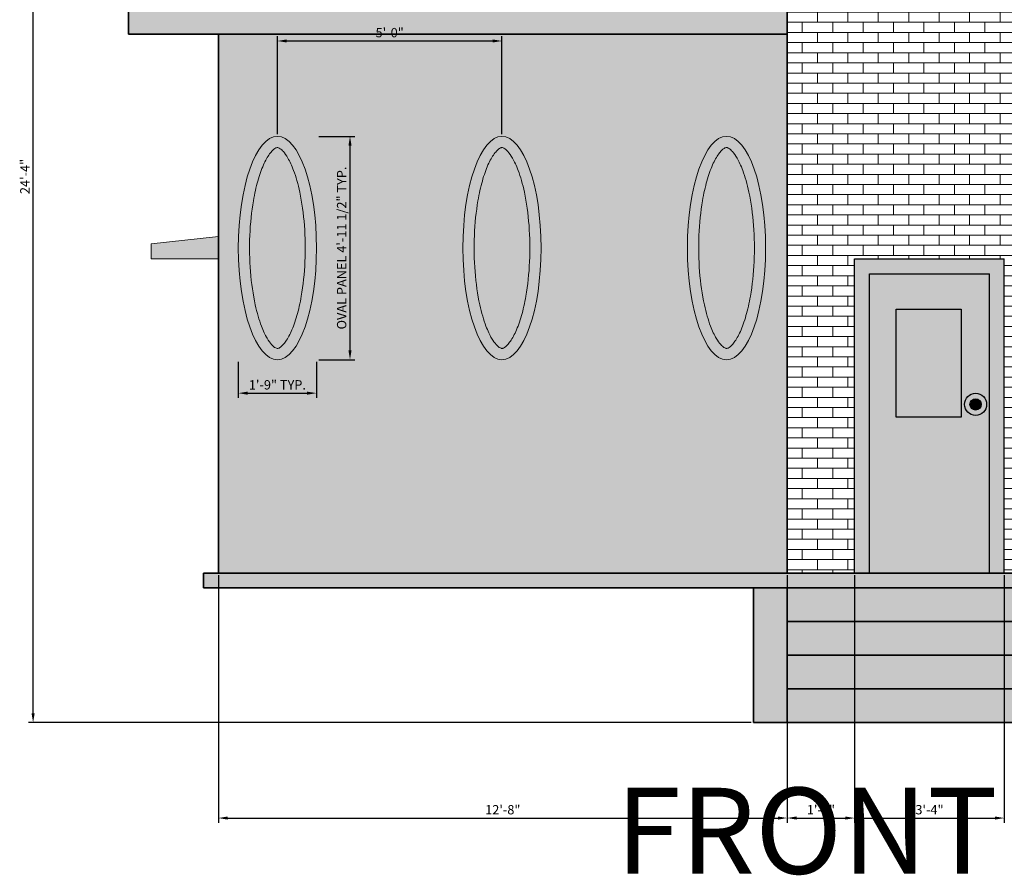
# Model space of a CAD drawing. Units: inches. Extents: x 4878 to 9282, y 5367 to 6617.
# Tile 1 of 14: x 4936 to 5199, y 5367 to 5596. Entities that reach past the tile are written whole.
import ezdxf

# ---------------------------------------------------------------- set-up
doc = ezdxf.new("R2010")
doc.units = ezdxf.units.IN
for name, color, linetype, lineweight in [('A-ANNO-DIMS', 2, 'Continuous', 18), ('A-ANNO-TITL', 3, 'Continuous', 30), ('A-ELEV', 7, 'Continuous', 35), ('A-ELEV-DOOR', 3, 'Continuous', 25), ('A-ELEV-TRIM', 7, 'Continuous', 20)]:
    doc.layers.add(name, color=color, linetype=linetype, lineweight=lineweight)
for name, color, linetype, lineweight, true_color in [('A-ELEV-BASE-PATT', 252, 'Continuous', 13, 0x939598), ('A-ELEV-CLAD-PATT', 215, 'Continuous', 13, 0xa953a0), ('A-ELEV-DOOR-PATT', 37, 'Continuous', 13, 0x7f5f3f), ('A-ELEV-METL-PATT', 252, 'Continuous', 13, 0x939598), ('A-ELEV-PANL-PATT', 41, 'Continuous', 13, 0xf4ee51), ('A-ELEV-TRIM-PATT', 11, 'Continuous', 13, 0xf27172), ('A-ELEV-WALL-PATT', 9, 'Continuous', 13, 0xafd9aa)]:
    doc.layers.add(name, color=color, linetype=linetype, lineweight=lineweight, true_color=true_color)
doc.styles.get("Standard").update_dxf_attribs({"font": 'arial.ttf'})
doc.dimstyles.new('ISO-25', dxfattribs={"dimtxt": 2.5, "dimasz": 2.5, "dimexe": 1.25, "dimexo": 0.625, "dimtad": 1, "dimdec": 0, "dimlunit": 3, "dimtxsty": 'Standard', "dimcen": 2.5, "dimadec": 0, "dimazin": 0, "dimtfac": 1, "dimtdec": 0, "dimtmove": 0, "dimatfit": 3, "dimfxl": 1, "dimarcsym": 0})

# ---------------------------------------------------------------- blocks, each defined once
blk = doc.blocks.new('FACADE-OVAL-PANEL')
blk.add_ellipse((10.45, 29.85), major_axis=(0, -29.85), ratio=0.35)
blk.add_open_spline([(10.45, 3), (10.51, 3), (10.59, 3.01), (10.8, 3.08), (10.94, 3.14), (11.29, 3.36), (11.5, 3.53), (11.97, 3.99), (12.23, 4.29), (13.03, 5.37), (13.6, 6.35), (14.68, 8.75), (15.19, 10.18), (16.1, 13.36), (16.5, 15.12), (17.33, 19.86), (17.67, 23), (17.95, 29.42), (17.91, 32.7), (17.43, 39.02), (17.01, 42.06), (15.97, 46.94), (15.4, 48.9), (14.3, 51.87), (13.77, 52.99), (12.83, 54.61), (12.41, 55.2), (11.72, 55.97), (11.44, 56.22), (11.01, 56.52), (10.85, 56.6), (10.62, 56.68), (10.54, 56.69), (10.39, 56.7), (10.32, 56.69), (10.11, 56.63), (9.97, 56.57), (9.61, 56.34), (9.39, 56.16), (8.9, 55.68), (8.63, 55.37), (7.82, 54.26), (7.25, 53.26), (6.17, 50.82), (5.65, 49.37), (4.75, 46.15), (4.35, 44.37), (3.53, 39.59), (3.2, 36.44), (2.94, 30), (3, 26.71), (3.49, 20.39), (3.93, 17.36), (4.99, 12.53), (5.55, 10.61), (6.65, 7.7), (7.17, 6.6), (8.1, 5.01), (8.52, 4.45), (9.2, 3.69), (9.48, 3.45), (9.94, 3.14), (10.11, 3.07), (10.32, 3.01), (10.38, 3), (10.45, 3)], degree=3, knots=[0, 0, 0, 0, 0.110339, 0.110339, 0.220677, 0.220677, 0.331016, 0.331016, 0.441355, 0.441355, 0.663086, 0.663086, 0.884817, 0.884817, 1.106548, 1.106548, 1.444005, 1.444005, 1.781462, 1.781462, 2.118918, 2.118918, 2.388345, 2.388345, 2.598365, 2.598365, 2.76649, 2.76649, 2.902512, 2.902512, 3.016819, 3.016819, 3.131125, 3.131125, 3.245431, 3.245431, 3.359737, 3.359737, 3.474044, 3.474044, 3.58835, 3.58835, 3.811147, 3.811147, 4.033944, 4.033944, 4.256741, 4.256741, 4.594929, 4.594929, 4.933117, 4.933117, 5.271305, 5.271305, 5.538007, 5.538007, 5.746376, 5.746376, 5.91327, 5.91327, 6.048323, 6.048323, 6.183376, 6.183376, 6.283185, 6.283185, 6.283185, 6.283185])
blk = doc.blocks.new('*D49')
at = {"layer": 'A-ANNO-DIMS', "color": 0, "lineweight": -2, "transparency": 16777216}
for p, q in [((5015.83, 5564.48), (5025.4, 5564.48)), ((5024.15, 5507.29), (5024.15, 5561.98)), ((5015.83, 5504.79), (5025.4, 5504.79))]:
    blk.add_line(p, q, dxfattribs=at)
at = {"layer": 'A-ANNO-DIMS', "color": 0, "transparency": 16777216}
for points in [[(5023.74, 5561.98), (5024.57, 5561.98), (5024.15, 5564.48)], [(5023.74, 5507.29), (5024.57, 5507.29), (5024.15, 5504.79)]]:
    blk.add_solid(points, dxfattribs=at)
at = {"layer": 'Defpoints', "color": 0, "transparency": 16777216}
for p in [(5015.2, 5564.48), (5024.15, 5564.48), (5015.2, 5504.79)]:
    blk.add_point(p, dxfattribs=at)
at = {"layer": 'A-ANNO-DIMS', "color": 0, "transparency": 16777216, "insert": (5022.24, 5534.64), "char_height": 2.5, "attachment_point": 5, "rotation": 90}
blk.add_mtext('OVAL PANEL 4\'-11 1/2" TYP.', dxfattribs=at)
blk = doc.blocks.new('*D50')
at = {"layer": 'A-ANNO-DIMS', "color": 0, "lineweight": -2, "transparency": 16777216}
for p, q in [((4994.31, 5504.17), (4994.31, 5494.59)), ((5015.2, 5504.17), (5015.2, 5494.59)), ((4996.81, 5495.84), (5012.7, 5495.84))]:
    blk.add_line(p, q, dxfattribs=at)
at = {"layer": 'A-ANNO-DIMS', "color": 0, "transparency": 16777216}
for points in [[(4996.81, 5496.25), (4996.81, 5495.42), (4994.31, 5495.84)], [(5012.7, 5496.25), (5012.7, 5495.42), (5015.2, 5495.84)]]:
    blk.add_solid(points, dxfattribs=at)
at = {"layer": 'Defpoints', "color": 0, "transparency": 16777216}
for p in [(4994.31, 5504.79), (5015.2, 5504.79), (5015.2, 5495.84)]:
    blk.add_point(p, dxfattribs=at)
at = {"layer": 'A-ANNO-DIMS', "color": 0, "transparency": 16777216, "insert": (5004.75, 5497.74), "char_height": 2.5, "attachment_point": 5}
blk.add_mtext('1\'-9" TYP.', dxfattribs=at)
blk = doc.blocks.new('*D89')
at = {"layer": 'A-ANNO-DIMS', "color": 0, "lineweight": -2, "transparency": 16777216}
for p, q in [((5116.35, 5699.76), (4938.23, 5699.76)), ((4939.48, 5410.26), (4939.48, 5697.26)), ((5131.35, 5407.76), (4938.23, 5407.76))]:
    blk.add_line(p, q, dxfattribs=at)
at = {"layer": 'A-ANNO-DIMS', "color": 0, "transparency": 16777216}
for points in [[(4939.06, 5697.26), (4939.89, 5697.26), (4939.48, 5699.76)], [(4939.06, 5410.26), (4939.89, 5410.26), (4939.48, 5407.76)]]:
    blk.add_solid(points, dxfattribs=at)
at = {"layer": 'Defpoints', "color": 0, "transparency": 16777216}
for p in [(4939.48, 5699.76), (5116.98, 5699.76), (5131.98, 5407.76)]:
    blk.add_point(p, dxfattribs=at)
at = {"layer": 'A-ANNO-DIMS', "color": 0, "transparency": 16777216, "insert": (4937.6, 5553.76), "char_height": 2.5, "attachment_point": 5, "rotation": 90}
blk.add_mtext('24\'-4"', dxfattribs=at)
blk = doc.blocks.new('*D90')
at = {"layer": 'A-ANNO-DIMS', "color": 0, "lineweight": -2, "transparency": 16777216}
for p, q in [((4988.98, 5447.14), (4988.98, 5381.01)), ((5140.98, 5447.14), (5140.98, 5381.01)), ((4991.48, 5382.26), (5138.48, 5382.26))]:
    blk.add_line(p, q, dxfattribs=at)
at = {"layer": 'A-ANNO-DIMS', "color": 0, "transparency": 16777216}
for points in [[(4991.48, 5382.68), (4991.48, 5381.84), (4988.98, 5382.26)], [(5138.48, 5382.68), (5138.48, 5381.84), (5140.98, 5382.26)]]:
    blk.add_solid(points, dxfattribs=at)
at = {"layer": 'Defpoints', "color": 0, "transparency": 16777216}
for p in [(4988.98, 5447.76), (5140.98, 5447.76), (5140.98, 5382.26)]:
    blk.add_point(p, dxfattribs=at)
at = {"layer": 'A-ANNO-DIMS', "color": 0, "transparency": 16777216, "insert": (5064.98, 5384.16), "char_height": 2.5, "attachment_point": 5}
blk.add_mtext('12\'-8"', dxfattribs=at)
blk = doc.blocks.new('*D91')
at = {"layer": 'A-ANNO-DIMS', "color": 0, "lineweight": -2, "transparency": 16777216}
for p, q in [((5140.98, 5447.14), (5140.98, 5381.01)), ((5158.98, 5447.14), (5158.98, 5381.01)), ((5143.48, 5382.26), (5156.48, 5382.26))]:
    blk.add_line(p, q, dxfattribs=at)
at = {"layer": 'A-ANNO-DIMS', "color": 0, "transparency": 16777216}
for points in [[(5143.48, 5382.68), (5143.48, 5381.84), (5140.98, 5382.26)], [(5156.48, 5382.68), (5156.48, 5381.84), (5158.98, 5382.26)]]:
    blk.add_solid(points, dxfattribs=at)
at = {"layer": 'Defpoints', "color": 0, "transparency": 16777216}
for p in [(5140.98, 5447.76), (5158.98, 5447.76), (5158.98, 5382.26)]:
    blk.add_point(p, dxfattribs=at)
at = {"layer": 'A-ANNO-DIMS', "color": 0, "transparency": 16777216, "insert": (5149.98, 5384.16), "char_height": 2.5, "attachment_point": 5}
blk.add_mtext('1\'-6"', dxfattribs=at)
blk = doc.blocks.new('*D92')
at = {"layer": 'A-ANNO-DIMS', "color": 0, "lineweight": -2, "transparency": 16777216}
for p, q in [((5158.98, 5447.14), (5158.98, 5381.01)), ((5198.98, 5447.14), (5198.98, 5381.01)), ((5161.48, 5382.26), (5196.48, 5382.26))]:
    blk.add_line(p, q, dxfattribs=at)
at = {"layer": 'A-ANNO-DIMS', "color": 0, "transparency": 16777216}
for points in [[(5161.48, 5382.68), (5161.48, 5381.84), (5158.98, 5382.26)], [(5196.48, 5382.68), (5196.48, 5381.84), (5198.98, 5382.26)]]:
    blk.add_solid(points, dxfattribs=at)
at = {"layer": 'Defpoints', "color": 0, "transparency": 16777216}
for p in [(5158.98, 5447.76), (5198.98, 5447.76), (5198.98, 5382.26)]:
    blk.add_point(p, dxfattribs=at)
at = {"layer": 'A-ANNO-DIMS', "color": 0, "transparency": 16777216, "insert": (5178.98, 5384.16), "char_height": 2.5, "attachment_point": 5}
blk.add_mtext('3\'-4"', dxfattribs=at)
blk = doc.blocks.new('*D99')
at = {"layer": 'A-ANNO-DIMS', "color": 0, "lineweight": -2, "transparency": 16777216}
for p, q in [((5004.75, 5565.11), (5004.75, 5591.23)), ((5064.75, 5565.11), (5064.75, 5591.23)), ((5007.25, 5589.98), (5062.25, 5589.98))]:
    blk.add_line(p, q, dxfattribs=at)
at = {"layer": 'A-ANNO-DIMS', "color": 0, "transparency": 16777216}
for points in [[(5007.25, 5590.4), (5007.25, 5589.57), (5004.75, 5589.98)], [(5062.25, 5590.4), (5062.25, 5589.57), (5064.75, 5589.98)]]:
    blk.add_solid(points, dxfattribs=at)
at = {"layer": 'Defpoints', "color": 0, "transparency": 16777216}
for p in [(5064.75, 5589.98), (5004.75, 5564.48), (5064.75, 5564.48)]:
    blk.add_point(p, dxfattribs=at)
at = {"layer": 'A-ANNO-DIMS', "color": 0, "transparency": 16777216, "insert": (5034.75, 5591.89), "char_height": 2.5, "attachment_point": 5}
blk.add_mtext('5\'-0"', dxfattribs=at)

msp = doc.modelspace()

# ---------------------------------------------------------------- hatches: boundary and pattern name
at = {"layer": 'A-ELEV-BASE-PATT'}
h = msp.add_hatch(color=256, dxfattribs=at)
h.dxf.hatch_style = 1
h.paths.add_polyline_path([(4984.98, 5447.76), (4984.98, 5443.76), (5449.48, 5443.76), (5449.48, 5447.76)])
h = msp.add_hatch(color=256, dxfattribs=at)
h.dxf.hatch_style = 1
h.paths.add_polyline_path([(5140.98, 5443.76), (5131.98, 5443.76), (5131.98, 5407.76), (5140.98, 5407.76)])
h.paths.add_polyline_path([(5302.48, 5407.76), (5311.48, 5407.76), (5311.48, 5443.76), (5302.48, 5443.76)])
h = msp.add_hatch(color=256, dxfattribs=at)
h.dxf.hatch_style = 1
h.paths.add_polyline_path([(5302.48, 5434.76), (5302.48, 5443.76), (5140.98, 5443.76), (5140.98, 5434.76)])
h.paths.add_polyline_path([(5302.48, 5416.76), (5302.48, 5425.76), (5140.98, 5425.76), (5140.98, 5416.76)])
h = msp.add_hatch(color=256, dxfattribs=at)
h.dxf.hatch_style = 1
h.paths.add_polyline_path([(5302.48, 5407.76), (5302.48, 5416.76), (5140.98, 5416.76), (5140.98, 5407.76)])
h.paths.add_polyline_path([(5140.98, 5434.76), (5140.98, 5425.76), (5302.48, 5425.76), (5302.48, 5434.76)])
at = {"layer": 'A-ELEV-CLAD-PATT'}
h = msp.add_hatch(dxfattribs=at)
h.set_pattern_fill('AR-BRSTD', color=256, scale=0.04)
h.set_pattern_definition([(0, (-2235.2307, 189.171), (0, 2.709672), []), (90, (-2235.2307, 189.171), (-4.064, 2.709672), [2.709672, -2.709672])])
h.paths.add_polyline_path([(5140.98, 5447.76), (5158.98, 5447.76), (5158.98, 5531.76), (5198.98, 5531.76), (5198.98, 5447.76), (5302.48, 5447.76), (5302.48, 5693.76), (5140.98, 5693.76)])
h.paths.add_polyline_path([(5225.95, 5537.76), (5279.95, 5537.76), (5279.95, 5531.76), (5273.95, 5531.76), (5273.95, 5495.76), (5231.95, 5495.76), (5231.95, 5531.76), (5225.95, 5531.76)], flags=16)
h.paths.add_polyline_path([(5234.95, 5528.76), (5270.95, 5528.76), (5270.95, 5498.76), (5234.95, 5498.76)], flags=0)
at = {"layer": 'A-ELEV-DOOR-PATT'}
h = msp.add_hatch(color=256, dxfattribs=at)
h.dxf.hatch_style = 1
h.paths.add_polyline_path([(5162.98, 5527.76), (5194.98, 5527.76), (5194.98, 5447.76), (5198.98, 5447.76), (5198.98, 5531.76), (5158.98, 5531.76), (5158.98, 5447.76), (5162.98, 5447.76)])
h.paths.add_polyline_path([(5170.08, 5489.4), (5187.41, 5489.4), (5187.41, 5518.26), (5170.08, 5518.26)], flags=17)
h = msp.add_hatch(color=256, dxfattribs=at)
h.dxf.hatch_style = 1
h.paths.add_polyline_path([(5162.98, 5527.76), (5162.98, 5447.76), (5194.98, 5447.76), (5194.98, 5527.76)])
h.paths.add_polyline_path([(5187.41, 5518.26), (5187.41, 5489.4), (5170.08, 5489.4), (5170.08, 5518.26)], flags=16)
h.paths.add_polyline_path([(5194.25, 5492.84, -1), (5188.34, 5492.84, -1)], flags=16)
h.paths.add_polyline_path([(5192.82, 5492.84, -1), (5189.78, 5492.84, -1)], flags=0)
at = {"layer": 'A-ELEV-METL-PATT'}
h = msp.add_hatch(color=256, dxfattribs=at)
h.dxf.hatch_style = 1
h.paths.add_polyline_path([(5188.34, 5492.84, 1), (5194.25, 5492.84, 1)])
h.paths.add_polyline_path([(5192.82, 5492.84, -1), (5189.78, 5492.84, -1)], flags=16)
h = msp.add_hatch(color=256, dxfattribs=at)
h.dxf.hatch_style = 1
h.paths.add_polyline_path([(5192.82, 5492.84, 1), (5189.78, 5492.84, 1)])
at = {"layer": 'A-ELEV-PANL-PATT'}
h = msp.add_hatch(color=256, dxfattribs=at)
h.dxf.hatch_style = 1
edge = h.paths.add_edge_path()
edge.add_spline(control_points=[(5004.75, 5507.79), (5004.82, 5507.79), (5004.89, 5507.8), (5005.1, 5507.87), (5005.24, 5507.93), (5005.6, 5508.15), (5005.81, 5508.32), (5006.28, 5508.78), (5006.54, 5509.08), (5007.34, 5510.16), (5007.91, 5511.14), (5008.99, 5513.54), (5009.5, 5514.97), (5010.41, 5518.15), (5010.81, 5519.91), (5011.64, 5524.65), (5011.98, 5527.79), (5012.26, 5534.21), (5012.21, 5537.49), (5011.74, 5543.82), (5011.32, 5546.85), (5010.27, 5551.73), (5009.71, 5553.69), (5008.6, 5556.66), (5008.08, 5557.78), (5007.14, 5559.41), (5006.72, 5559.99), (5006.03, 5560.76), (5005.75, 5561.01), (5005.32, 5561.31), (5005.16, 5561.39), (5004.92, 5561.47), (5004.85, 5561.48), (5004.7, 5561.49), (5004.63, 5561.48), (5004.42, 5561.42), (5004.28, 5561.36), (5003.92, 5561.13), (5003.7, 5560.96), (5003.21, 5560.47), (5002.94, 5560.16), (5002.12, 5559.05), (5001.55, 5558.05), (5000.47, 5555.61), (4999.96, 5554.17), (4999.05, 5550.94), (4998.66, 5549.16), (4997.84, 5544.38), (4997.51, 5541.23), (4997.24, 5534.79), (4997.3, 5531.5), (4997.8, 5525.18), (4998.24, 5522.15), (4999.29, 5517.32), (4999.86, 5515.4), (5000.96, 5512.49), (5001.48, 5511.39), (5002.41, 5509.8), (5002.83, 5509.24), (5003.51, 5508.48), (5003.79, 5508.24), (5004.24, 5507.93), (5004.42, 5507.86), (5004.63, 5507.8), (5004.69, 5507.79), (5004.75, 5507.79)], knot_values=[0, 0, 0, 0, 0.110339, 0.110339, 0.220677, 0.220677, 0.331016, 0.331016, 0.441355, 0.441355, 0.663086, 0.663086, 0.884817, 0.884817, 1.106548, 1.106548, 1.444005, 1.444005, 1.781462, 1.781462, 2.118918, 2.118918, 2.388345, 2.388345, 2.598365, 2.598365, 2.76649, 2.76649, 2.902512, 2.902512, 3.016819, 3.016819, 3.131125, 3.131125, 3.245431, 3.245431, 3.359737, 3.359737, 3.474044, 3.474044, 3.58835, 3.58835, 3.811147, 3.811147, 4.033944, 4.033944, 4.256741, 4.256741, 4.594929, 4.594929, 4.933117, 4.933117, 5.271305, 5.271305, 5.538007, 5.538007, 5.746376, 5.746376, 5.91327, 5.91327, 6.048323, 6.048323, 6.183376, 6.183376, 6.283185, 6.283185, 6.283185, 6.283185], degree=3, periodic=0)
edge = h.paths.add_edge_path()
edge.add_spline(control_points=[(5064.75, 5507.79), (5064.82, 5507.79), (5064.89, 5507.8), (5065.1, 5507.87), (5065.24, 5507.93), (5065.6, 5508.15), (5065.81, 5508.32), (5066.28, 5508.78), (5066.54, 5509.08), (5067.34, 5510.16), (5067.91, 5511.14), (5068.99, 5513.54), (5069.5, 5514.97), (5070.41, 5518.15), (5070.81, 5519.91), (5071.64, 5524.65), (5071.98, 5527.79), (5072.26, 5534.21), (5072.21, 5537.49), (5071.74, 5543.82), (5071.32, 5546.85), (5070.27, 5551.73), (5069.71, 5553.69), (5068.6, 5556.66), (5068.08, 5557.78), (5067.14, 5559.41), (5066.72, 5559.99), (5066.03, 5560.76), (5065.75, 5561.01), (5065.32, 5561.31), (5065.16, 5561.39), (5064.92, 5561.47), (5064.85, 5561.48), (5064.7, 5561.49), (5064.63, 5561.48), (5064.42, 5561.42), (5064.28, 5561.36), (5063.92, 5561.13), (5063.7, 5560.96), (5063.21, 5560.47), (5062.94, 5560.16), (5062.12, 5559.05), (5061.55, 5558.05), (5060.47, 5555.61), (5059.96, 5554.17), (5059.05, 5550.94), (5058.66, 5549.16), (5057.84, 5544.38), (5057.51, 5541.23), (5057.24, 5534.79), (5057.3, 5531.5), (5057.8, 5525.18), (5058.24, 5522.15), (5059.29, 5517.32), (5059.86, 5515.4), (5060.96, 5512.49), (5061.48, 5511.39), (5062.41, 5509.8), (5062.83, 5509.24), (5063.51, 5508.48), (5063.79, 5508.24), (5064.24, 5507.93), (5064.42, 5507.86), (5064.63, 5507.8), (5064.69, 5507.79), (5064.75, 5507.79)], knot_values=[0, 0, 0, 0, 0.110339, 0.110339, 0.220677, 0.220677, 0.331016, 0.331016, 0.441355, 0.441355, 0.663086, 0.663086, 0.884817, 0.884817, 1.106548, 1.106548, 1.444005, 1.444005, 1.781462, 1.781462, 2.118918, 2.118918, 2.388345, 2.388345, 2.598365, 2.598365, 2.76649, 2.76649, 2.902512, 2.902512, 3.016819, 3.016819, 3.131125, 3.131125, 3.245431, 3.245431, 3.359737, 3.359737, 3.474044, 3.474044, 3.58835, 3.58835, 3.811147, 3.811147, 4.033944, 4.033944, 4.256741, 4.256741, 4.594929, 4.594929, 4.933117, 4.933117, 5.271305, 5.271305, 5.538007, 5.538007, 5.746376, 5.746376, 5.91327, 5.91327, 6.048323, 6.048323, 6.183376, 6.183376, 6.283185, 6.283185, 6.283185, 6.283185], degree=3, periodic=0)
edge = h.paths.add_edge_path()
edge.add_spline(control_points=[(5124.75, 5507.79), (5124.82, 5507.79), (5124.89, 5507.8), (5125.1, 5507.87), (5125.24, 5507.93), (5125.6, 5508.15), (5125.81, 5508.32), (5126.28, 5508.78), (5126.54, 5509.08), (5127.34, 5510.16), (5127.91, 5511.14), (5128.99, 5513.54), (5129.5, 5514.97), (5130.41, 5518.15), (5130.81, 5519.91), (5131.64, 5524.65), (5131.98, 5527.79), (5132.26, 5534.21), (5132.21, 5537.49), (5131.74, 5543.82), (5131.32, 5546.85), (5130.27, 5551.73), (5129.71, 5553.69), (5128.6, 5556.66), (5128.08, 5557.78), (5127.14, 5559.41), (5126.72, 5559.99), (5126.03, 5560.76), (5125.75, 5561.01), (5125.32, 5561.31), (5125.16, 5561.39), (5124.92, 5561.47), (5124.85, 5561.48), (5124.7, 5561.49), (5124.63, 5561.48), (5124.42, 5561.42), (5124.28, 5561.36), (5123.92, 5561.13), (5123.7, 5560.96), (5123.21, 5560.47), (5122.94, 5560.16), (5122.12, 5559.05), (5121.55, 5558.05), (5120.47, 5555.61), (5119.96, 5554.17), (5119.05, 5550.94), (5118.66, 5549.16), (5117.84, 5544.38), (5117.51, 5541.23), (5117.24, 5534.79), (5117.3, 5531.5), (5117.8, 5525.18), (5118.24, 5522.15), (5119.29, 5517.32), (5119.86, 5515.4), (5120.96, 5512.49), (5121.48, 5511.39), (5122.41, 5509.8), (5122.83, 5509.24), (5123.51, 5508.48), (5123.79, 5508.24), (5124.24, 5507.93), (5124.42, 5507.86), (5124.63, 5507.8), (5124.69, 5507.79), (5124.75, 5507.79)], knot_values=[0, 0, 0, 0, 0.110339, 0.110339, 0.220677, 0.220677, 0.331016, 0.331016, 0.441355, 0.441355, 0.663086, 0.663086, 0.884817, 0.884817, 1.106548, 1.106548, 1.444005, 1.444005, 1.781462, 1.781462, 2.118918, 2.118918, 2.388345, 2.388345, 2.598365, 2.598365, 2.76649, 2.76649, 2.902512, 2.902512, 3.016819, 3.016819, 3.131125, 3.131125, 3.245431, 3.245431, 3.359737, 3.359737, 3.474044, 3.474044, 3.58835, 3.58835, 3.811147, 3.811147, 4.033944, 4.033944, 4.256741, 4.256741, 4.594929, 4.594929, 4.933117, 4.933117, 5.271305, 5.271305, 5.538007, 5.538007, 5.746376, 5.746376, 5.91327, 5.91327, 6.048323, 6.048323, 6.183376, 6.183376, 6.283185, 6.283185, 6.283185, 6.283185], degree=3, periodic=0)
at = {"layer": 'A-ELEV-TRIM-PATT'}
h = msp.add_hatch(color=256, dxfattribs=at)
h.dxf.hatch_style = 1
h.paths.add_polyline_path([(5140.98, 5591.76), (5140.98, 5597.76), (4964.98, 5597.76), (4964.98, 5591.76)])
h.paths.add_polyline_path([(5112.98, 5633.76), (5112.98, 5637.76), (5095.98, 5637.76), (5095.98, 5633.76)])
h.paths.add_polyline_path([(5035.98, 5637.76), (5035.98, 5633.76), (5052.98, 5633.76), (5052.98, 5637.76)])
h.paths.add_polyline_path([(4975.98, 5637.76), (4975.98, 5633.76), (4992.98, 5633.76), (4992.98, 5637.76)])
h.paths.add_polyline_path([(5116.98, 5699.76), (5116.98, 5693.76), (5326.48, 5693.76), (5326.48, 5699.76)])
h.paths.add_polyline_path([(5321.48, 5637.76), (5321.48, 5633.76), (5338.48, 5633.76), (5338.48, 5637.76)])
h.paths.add_polyline_path([(5381.48, 5637.76), (5381.48, 5633.76), (5398.48, 5633.76), (5398.48, 5637.76)])
h.paths.add_polyline_path([(5441.48, 5637.76), (5441.48, 5633.76), (5458.48, 5633.76), (5458.48, 5637.76)])
h.paths.add_polyline_path([(5469.48, 5591.76), (5469.48, 5597.76), (5302.48, 5597.76), (5302.48, 5591.76)])
h.paths.add_polyline_path([(5346.98, 5537.76), (5346.98, 5531.76), (5400.98, 5531.76), (5400.98, 5537.76)])
h.paths.add_polyline_path([(5279.95, 5531.76), (5279.95, 5537.76), (5225.95, 5537.76), (5225.95, 5531.76)])
h = msp.add_hatch(color=256, dxfattribs=at)
h.dxf.hatch_style = 1
edge = h.paths.add_edge_path()
edge.add_ellipse((5004.75, 5534.64), major_axis=(0, -29.85), ratio=0.35, start_angle=0, end_angle=360)
edge = h.paths.add_edge_path(flags=16)
edge.add_spline(control_points=[(5004.75, 5507.79), (5004.82, 5507.79), (5004.89, 5507.8), (5005.1, 5507.87), (5005.24, 5507.93), (5005.6, 5508.15), (5005.81, 5508.32), (5006.28, 5508.78), (5006.54, 5509.08), (5007.34, 5510.16), (5007.91, 5511.14), (5008.99, 5513.54), (5009.5, 5514.97), (5010.41, 5518.15), (5010.81, 5519.91), (5011.64, 5524.65), (5011.98, 5527.79), (5012.26, 5534.21), (5012.21, 5537.49), (5011.74, 5543.82), (5011.32, 5546.85), (5010.27, 5551.73), (5009.71, 5553.69), (5008.6, 5556.66), (5008.08, 5557.78), (5007.14, 5559.41), (5006.72, 5559.99), (5006.03, 5560.76), (5005.75, 5561.01), (5005.32, 5561.31), (5005.16, 5561.39), (5004.92, 5561.47), (5004.85, 5561.48), (5004.7, 5561.49), (5004.63, 5561.48), (5004.42, 5561.42), (5004.28, 5561.36), (5003.92, 5561.13), (5003.7, 5560.96), (5003.21, 5560.47), (5002.94, 5560.16), (5002.12, 5559.05), (5001.55, 5558.05), (5000.47, 5555.61), (4999.96, 5554.17), (4999.05, 5550.94), (4998.66, 5549.16), (4997.84, 5544.38), (4997.51, 5541.23), (4997.24, 5534.79), (4997.3, 5531.5), (4997.8, 5525.18), (4998.24, 5522.15), (4999.29, 5517.32), (4999.86, 5515.4), (5000.96, 5512.49), (5001.48, 5511.39), (5002.41, 5509.8), (5002.83, 5509.24), (5003.51, 5508.48), (5003.79, 5508.24), (5004.24, 5507.93), (5004.42, 5507.86), (5004.63, 5507.8), (5004.69, 5507.79), (5004.75, 5507.79)], knot_values=[0, 0, 0, 0, 0.110339, 0.110339, 0.220677, 0.220677, 0.331016, 0.331016, 0.441355, 0.441355, 0.663086, 0.663086, 0.884817, 0.884817, 1.106548, 1.106548, 1.444005, 1.444005, 1.781462, 1.781462, 2.118918, 2.118918, 2.388345, 2.388345, 2.598365, 2.598365, 2.76649, 2.76649, 2.902512, 2.902512, 3.016819, 3.016819, 3.131125, 3.131125, 3.245431, 3.245431, 3.359737, 3.359737, 3.474044, 3.474044, 3.58835, 3.58835, 3.811147, 3.811147, 4.033944, 4.033944, 4.256741, 4.256741, 4.594929, 4.594929, 4.933117, 4.933117, 5.271305, 5.271305, 5.538007, 5.538007, 5.746376, 5.746376, 5.91327, 5.91327, 6.048323, 6.048323, 6.183376, 6.183376, 6.283185, 6.283185, 6.283185, 6.283185], degree=3, periodic=0)
edge = h.paths.add_edge_path()
edge.add_ellipse((5064.75, 5534.64), major_axis=(0, -29.85), ratio=0.35, start_angle=0, end_angle=360)
edge = h.paths.add_edge_path(flags=16)
edge.add_spline(control_points=[(5064.75, 5507.79), (5064.82, 5507.79), (5064.89, 5507.8), (5065.1, 5507.87), (5065.24, 5507.93), (5065.6, 5508.15), (5065.81, 5508.32), (5066.28, 5508.78), (5066.54, 5509.08), (5067.34, 5510.16), (5067.91, 5511.14), (5068.99, 5513.54), (5069.5, 5514.97), (5070.41, 5518.15), (5070.81, 5519.91), (5071.64, 5524.65), (5071.98, 5527.79), (5072.26, 5534.21), (5072.21, 5537.49), (5071.74, 5543.82), (5071.32, 5546.85), (5070.27, 5551.73), (5069.71, 5553.69), (5068.6, 5556.66), (5068.08, 5557.78), (5067.14, 5559.41), (5066.72, 5559.99), (5066.03, 5560.76), (5065.75, 5561.01), (5065.32, 5561.31), (5065.16, 5561.39), (5064.92, 5561.47), (5064.85, 5561.48), (5064.7, 5561.49), (5064.63, 5561.48), (5064.42, 5561.42), (5064.28, 5561.36), (5063.92, 5561.13), (5063.7, 5560.96), (5063.21, 5560.47), (5062.94, 5560.16), (5062.12, 5559.05), (5061.55, 5558.05), (5060.47, 5555.61), (5059.96, 5554.17), (5059.05, 5550.94), (5058.66, 5549.16), (5057.84, 5544.38), (5057.51, 5541.23), (5057.24, 5534.79), (5057.3, 5531.5), (5057.8, 5525.18), (5058.24, 5522.15), (5059.29, 5517.32), (5059.86, 5515.4), (5060.96, 5512.49), (5061.48, 5511.39), (5062.41, 5509.8), (5062.83, 5509.24), (5063.51, 5508.48), (5063.79, 5508.24), (5064.24, 5507.93), (5064.42, 5507.86), (5064.63, 5507.8), (5064.69, 5507.79), (5064.75, 5507.79)], knot_values=[0, 0, 0, 0, 0.110339, 0.110339, 0.220677, 0.220677, 0.331016, 0.331016, 0.441355, 0.441355, 0.663086, 0.663086, 0.884817, 0.884817, 1.106548, 1.106548, 1.444005, 1.444005, 1.781462, 1.781462, 2.118918, 2.118918, 2.388345, 2.388345, 2.598365, 2.598365, 2.76649, 2.76649, 2.902512, 2.902512, 3.016819, 3.016819, 3.131125, 3.131125, 3.245431, 3.245431, 3.359737, 3.359737, 3.474044, 3.474044, 3.58835, 3.58835, 3.811147, 3.811147, 4.033944, 4.033944, 4.256741, 4.256741, 4.594929, 4.594929, 4.933117, 4.933117, 5.271305, 5.271305, 5.538007, 5.538007, 5.746376, 5.746376, 5.91327, 5.91327, 6.048323, 6.048323, 6.183376, 6.183376, 6.283185, 6.283185, 6.283185, 6.283185], degree=3, periodic=0)
edge = h.paths.add_edge_path()
edge.add_ellipse((5124.75, 5534.64), major_axis=(0, -29.85), ratio=0.35, start_angle=0, end_angle=360)
edge = h.paths.add_edge_path(flags=16)
edge.add_spline(control_points=[(5124.75, 5507.79), (5124.82, 5507.79), (5124.89, 5507.8), (5125.1, 5507.87), (5125.24, 5507.93), (5125.6, 5508.15), (5125.81, 5508.32), (5126.28, 5508.78), (5126.54, 5509.08), (5127.34, 5510.16), (5127.91, 5511.14), (5128.99, 5513.54), (5129.5, 5514.97), (5130.41, 5518.15), (5130.81, 5519.91), (5131.64, 5524.65), (5131.98, 5527.79), (5132.26, 5534.21), (5132.21, 5537.49), (5131.74, 5543.82), (5131.32, 5546.85), (5130.27, 5551.73), (5129.71, 5553.69), (5128.6, 5556.66), (5128.08, 5557.78), (5127.14, 5559.41), (5126.72, 5559.99), (5126.03, 5560.76), (5125.75, 5561.01), (5125.32, 5561.31), (5125.16, 5561.39), (5124.92, 5561.47), (5124.85, 5561.48), (5124.7, 5561.49), (5124.63, 5561.48), (5124.42, 5561.42), (5124.28, 5561.36), (5123.92, 5561.13), (5123.7, 5560.96), (5123.21, 5560.47), (5122.94, 5560.16), (5122.12, 5559.05), (5121.55, 5558.05), (5120.47, 5555.61), (5119.96, 5554.17), (5119.05, 5550.94), (5118.66, 5549.16), (5117.84, 5544.38), (5117.51, 5541.23), (5117.24, 5534.79), (5117.3, 5531.5), (5117.8, 5525.18), (5118.24, 5522.15), (5119.29, 5517.32), (5119.86, 5515.4), (5120.96, 5512.49), (5121.48, 5511.39), (5122.41, 5509.8), (5122.83, 5509.24), (5123.51, 5508.48), (5123.79, 5508.24), (5124.24, 5507.93), (5124.42, 5507.86), (5124.63, 5507.8), (5124.69, 5507.79), (5124.75, 5507.79)], knot_values=[0, 0, 0, 0, 0.110339, 0.110339, 0.220677, 0.220677, 0.331016, 0.331016, 0.441355, 0.441355, 0.663086, 0.663086, 0.884817, 0.884817, 1.106548, 1.106548, 1.444005, 1.444005, 1.781462, 1.781462, 2.118918, 2.118918, 2.388345, 2.388345, 2.598365, 2.598365, 2.76649, 2.76649, 2.902512, 2.902512, 3.016819, 3.016819, 3.131125, 3.131125, 3.245431, 3.245431, 3.359737, 3.359737, 3.474044, 3.474044, 3.58835, 3.58835, 3.811147, 3.811147, 4.033944, 4.033944, 4.256741, 4.256741, 4.594929, 4.594929, 4.933117, 4.933117, 5.271305, 5.271305, 5.538007, 5.538007, 5.746376, 5.746376, 5.91327, 5.91327, 6.048323, 6.048323, 6.183376, 6.183376, 6.283185, 6.283185, 6.283185, 6.283185], degree=3, periodic=0)
h = msp.add_hatch(color=256, dxfattribs=at)
h.dxf.hatch_style = 1
h.paths.add_polyline_path([(4988.98, 5537.76), (4970.98, 5535.76), (4970.98, 5531.76), (4988.98, 5531.76)])
at = {"layer": 'A-ELEV-WALL-PATT'}
h = msp.add_hatch(color=256, dxfattribs=at)
h.dxf.hatch_style = 1
h.paths.add_polyline_path([(5140.98, 5591.76), (4988.98, 5591.76), (4988.98, 5447.76), (5140.98, 5447.76)])
edge = h.paths.add_edge_path(flags=16)
edge.add_ellipse((5124.75, 5534.64), major_axis=(0, -29.85), ratio=0.35, start_angle=0, end_angle=360)
edge = h.paths.add_edge_path(flags=16)
edge.add_ellipse((5064.75, 5534.64), major_axis=(0, -29.85), ratio=0.35, start_angle=0, end_angle=360)
edge = h.paths.add_edge_path(flags=0)
edge.add_spline(control_points=[(5124.75, 5507.79), (5124.82, 5507.79), (5124.89, 5507.8), (5125.1, 5507.87), (5125.24, 5507.93), (5125.6, 5508.15), (5125.81, 5508.32), (5126.28, 5508.78), (5126.54, 5509.08), (5127.34, 5510.16), (5127.91, 5511.14), (5128.99, 5513.54), (5129.5, 5514.97), (5130.41, 5518.15), (5130.81, 5519.91), (5131.64, 5524.65), (5131.98, 5527.79), (5132.26, 5534.21), (5132.21, 5537.49), (5131.74, 5543.82), (5131.32, 5546.85), (5130.27, 5551.73), (5129.71, 5553.69), (5128.6, 5556.66), (5128.08, 5557.78), (5127.14, 5559.41), (5126.72, 5559.99), (5126.03, 5560.76), (5125.75, 5561.01), (5125.32, 5561.31), (5125.16, 5561.39), (5124.92, 5561.47), (5124.85, 5561.48), (5124.7, 5561.49), (5124.63, 5561.48), (5124.42, 5561.42), (5124.28, 5561.36), (5123.92, 5561.13), (5123.7, 5560.96), (5123.21, 5560.47), (5122.94, 5560.16), (5122.12, 5559.05), (5121.55, 5558.05), (5120.47, 5555.61), (5119.96, 5554.17), (5119.05, 5550.94), (5118.66, 5549.16), (5117.84, 5544.38), (5117.51, 5541.23), (5117.24, 5534.79), (5117.3, 5531.5), (5117.8, 5525.18), (5118.24, 5522.15), (5119.29, 5517.32), (5119.86, 5515.4), (5120.96, 5512.49), (5121.48, 5511.39), (5122.41, 5509.8), (5122.83, 5509.24), (5123.51, 5508.48), (5123.79, 5508.24), (5124.24, 5507.93), (5124.42, 5507.86), (5124.63, 5507.8), (5124.69, 5507.79), (5124.75, 5507.79)], knot_values=[0, 0, 0, 0, 0.110339, 0.110339, 0.220677, 0.220677, 0.331016, 0.331016, 0.441355, 0.441355, 0.663086, 0.663086, 0.884817, 0.884817, 1.106548, 1.106548, 1.444005, 1.444005, 1.781462, 1.781462, 2.118918, 2.118918, 2.388345, 2.388345, 2.598365, 2.598365, 2.76649, 2.76649, 2.902512, 2.902512, 3.016819, 3.016819, 3.131125, 3.131125, 3.245431, 3.245431, 3.359737, 3.359737, 3.474044, 3.474044, 3.58835, 3.58835, 3.811147, 3.811147, 4.033944, 4.033944, 4.256741, 4.256741, 4.594929, 4.594929, 4.933117, 4.933117, 5.271305, 5.271305, 5.538007, 5.538007, 5.746376, 5.746376, 5.91327, 5.91327, 6.048323, 6.048323, 6.183376, 6.183376, 6.283185, 6.283185, 6.283185, 6.283185], degree=3, periodic=0)
edge = h.paths.add_edge_path(flags=0)
edge.add_spline(control_points=[(5064.75, 5507.79), (5064.82, 5507.79), (5064.89, 5507.8), (5065.1, 5507.87), (5065.24, 5507.93), (5065.6, 5508.15), (5065.81, 5508.32), (5066.28, 5508.78), (5066.54, 5509.08), (5067.34, 5510.16), (5067.91, 5511.14), (5068.99, 5513.54), (5069.5, 5514.97), (5070.41, 5518.15), (5070.81, 5519.91), (5071.64, 5524.65), (5071.98, 5527.79), (5072.26, 5534.21), (5072.21, 5537.49), (5071.74, 5543.82), (5071.32, 5546.85), (5070.27, 5551.73), (5069.71, 5553.69), (5068.6, 5556.66), (5068.08, 5557.78), (5067.14, 5559.41), (5066.72, 5559.99), (5066.03, 5560.76), (5065.75, 5561.01), (5065.32, 5561.31), (5065.16, 5561.39), (5064.92, 5561.47), (5064.85, 5561.48), (5064.7, 5561.49), (5064.63, 5561.48), (5064.42, 5561.42), (5064.28, 5561.36), (5063.92, 5561.13), (5063.7, 5560.96), (5063.21, 5560.47), (5062.94, 5560.16), (5062.12, 5559.05), (5061.55, 5558.05), (5060.47, 5555.61), (5059.96, 5554.17), (5059.05, 5550.94), (5058.66, 5549.16), (5057.84, 5544.38), (5057.51, 5541.23), (5057.24, 5534.79), (5057.3, 5531.5), (5057.8, 5525.18), (5058.24, 5522.15), (5059.29, 5517.32), (5059.86, 5515.4), (5060.96, 5512.49), (5061.48, 5511.39), (5062.41, 5509.8), (5062.83, 5509.24), (5063.51, 5508.48), (5063.79, 5508.24), (5064.24, 5507.93), (5064.42, 5507.86), (5064.63, 5507.8), (5064.69, 5507.79), (5064.75, 5507.79)], knot_values=[0, 0, 0, 0, 0.110339, 0.110339, 0.220677, 0.220677, 0.331016, 0.331016, 0.441355, 0.441355, 0.663086, 0.663086, 0.884817, 0.884817, 1.106548, 1.106548, 1.444005, 1.444005, 1.781462, 1.781462, 2.118918, 2.118918, 2.388345, 2.388345, 2.598365, 2.598365, 2.76649, 2.76649, 2.902512, 2.902512, 3.016819, 3.016819, 3.131125, 3.131125, 3.245431, 3.245431, 3.359737, 3.359737, 3.474044, 3.474044, 3.58835, 3.58835, 3.811147, 3.811147, 4.033944, 4.033944, 4.256741, 4.256741, 4.594929, 4.594929, 4.933117, 4.933117, 5.271305, 5.271305, 5.538007, 5.538007, 5.746376, 5.746376, 5.91327, 5.91327, 6.048323, 6.048323, 6.183376, 6.183376, 6.283185, 6.283185, 6.283185, 6.283185], degree=3, periodic=0)
edge = h.paths.add_edge_path(flags=16)
edge.add_ellipse((5004.75, 5534.64), major_axis=(0, -29.85), ratio=0.35, start_angle=0, end_angle=360)
edge = h.paths.add_edge_path(flags=0)
edge.add_spline(control_points=[(5004.75, 5507.79), (5004.82, 5507.79), (5004.89, 5507.8), (5005.1, 5507.87), (5005.24, 5507.93), (5005.6, 5508.15), (5005.81, 5508.32), (5006.28, 5508.78), (5006.54, 5509.08), (5007.34, 5510.16), (5007.91, 5511.14), (5008.99, 5513.54), (5009.5, 5514.97), (5010.41, 5518.15), (5010.81, 5519.91), (5011.64, 5524.65), (5011.98, 5527.79), (5012.26, 5534.21), (5012.21, 5537.49), (5011.74, 5543.82), (5011.32, 5546.85), (5010.27, 5551.73), (5009.71, 5553.69), (5008.6, 5556.66), (5008.08, 5557.78), (5007.14, 5559.41), (5006.72, 5559.99), (5006.03, 5560.76), (5005.75, 5561.01), (5005.32, 5561.31), (5005.16, 5561.39), (5004.92, 5561.47), (5004.85, 5561.48), (5004.7, 5561.49), (5004.63, 5561.48), (5004.42, 5561.42), (5004.28, 5561.36), (5003.92, 5561.13), (5003.7, 5560.96), (5003.21, 5560.47), (5002.94, 5560.16), (5002.12, 5559.05), (5001.55, 5558.05), (5000.47, 5555.61), (4999.96, 5554.17), (4999.05, 5550.94), (4998.66, 5549.16), (4997.84, 5544.38), (4997.51, 5541.23), (4997.24, 5534.79), (4997.3, 5531.5), (4997.8, 5525.18), (4998.24, 5522.15), (4999.29, 5517.32), (4999.86, 5515.4), (5000.96, 5512.49), (5001.48, 5511.39), (5002.41, 5509.8), (5002.83, 5509.24), (5003.51, 5508.48), (5003.79, 5508.24), (5004.24, 5507.93), (5004.42, 5507.86), (5004.63, 5507.8), (5004.69, 5507.79), (5004.75, 5507.79)], knot_values=[0, 0, 0, 0, 0.110339, 0.110339, 0.220677, 0.220677, 0.331016, 0.331016, 0.441355, 0.441355, 0.663086, 0.663086, 0.884817, 0.884817, 1.106548, 1.106548, 1.444005, 1.444005, 1.781462, 1.781462, 2.118918, 2.118918, 2.388345, 2.388345, 2.598365, 2.598365, 2.76649, 2.76649, 2.902512, 2.902512, 3.016819, 3.016819, 3.131125, 3.131125, 3.245431, 3.245431, 3.359737, 3.359737, 3.474044, 3.474044, 3.58835, 3.58835, 3.811147, 3.811147, 4.033944, 4.033944, 4.256741, 4.256741, 4.594929, 4.594929, 4.933117, 4.933117, 5.271305, 5.271305, 5.538007, 5.538007, 5.746376, 5.746376, 5.91327, 5.91327, 6.048323, 6.048323, 6.183376, 6.183376, 6.283185, 6.283185, 6.283185, 6.283185], degree=3, periodic=0)

# ---------------------------------------------------------------- linework, layer by layer
at = {"layer": 'A-ELEV'}
for p, q in [((5140.98, 5693.76), (5140.98, 5447.76)), ((4964.98, 5597.76), (4964.98, 5591.76)), ((4964.98, 5591.76), (5140.98, 5591.76)), ((4988.98, 5591.76), (4988.98, 5447.76)), ((4984.98, 5447.76), (5449.48, 5447.76)), ((4984.98, 5447.76), (4984.98, 5443.76)), ((4984.98, 5443.76), (5449.48, 5443.76)), ((5131.98, 5407.76), (5131.98, 5443.76)), ((5140.98, 5443.76), (5140.98, 5407.76)), ((5140.98, 5434.76), (5302.48, 5434.76)), ((5140.98, 5425.76), (5302.48, 5425.76)), ((5140.98, 5416.76), (5302.48, 5416.76)), ((5131.98, 5407.76), (5311.48, 5407.76))]:
    msp.add_line(p, q, dxfattribs=at)
at = {"layer": 'A-ELEV-DOOR'}
for p, q in [((5158.98, 5447.76), (5158.98, 5531.76)), ((5158.98, 5531.76), (5198.98, 5531.76)), ((5198.98, 5447.76), (5198.98, 5531.76)), ((5162.98, 5527.76), (5194.98, 5527.76)), ((5162.98, 5447.76), (5162.98, 5527.76)), ((5194.98, 5447.76), (5194.98, 5527.76))]:
    msp.add_line(p, q, dxfattribs=at)
msp.add_lwpolyline([(5170.08, 5518.26), (5187.41, 5518.26), (5187.41, 5489.4), (5170.08, 5489.4)], close=True, dxfattribs=at)
for radius in [2.96, 1.52]:
    msp.add_circle((5191.3, 5492.84), radius, dxfattribs=at)
at = {"layer": 'A-ELEV-TRIM'}
for p, q in [((4970.98, 5535.76), (4988.98, 5537.76)), ((4970.98, 5531.76), (4970.98, 5535.76)), ((4988.98, 5531.76), (4970.98, 5531.76))]:
    msp.add_line(p, q, dxfattribs=at)

# ---------------------------------------------------------------- block references
for p in [(4994.31, 5504.79), (5054.31, 5504.79), (5114.31, 5504.79)]:
    msp.add_blockref('FACADE-OVAL-PANEL', p, dxfattribs=at)

# ---------------------------------------------------------------- texts
at = {"layer": 'A-ANNO-TITL', "insert": (5095.17, 5390.36), "char_height": 23, "attachment_point": 1}
msp.add_mtext_dynamic_manual_height_columns('FRONT ELEVATION', width=1356.1732, gutter_width=12.5, heights=[0], dxfattribs=at)

# ---------------------------------------------------------------- dimensions: what is measured, and where the dimension line sits
at = {"layer": 'A-ANNO-DIMS'}
dim = msp.add_linear_dim(base=(4939.48, 5699.76), p1=(5131.98, 5407.76), p2=(5116.98, 5699.76), angle=90, dimstyle='ISO-25', override={"dimdec": 1, "dimlfac": 1, "dimrnd": 0, "dimzin": 1, "dimdsep": 46, "dimlunit": 4, "dimfrac": 2}, dxfattribs=at)
dim.commit()
dim.dimension.update_dxf_attribs({"geometry": '*D89', "text_midpoint": (4937.6, 5553.76)})
for base, p1, p2, picture, middle in [((5064.75, 5589.98), (5004.75, 5564.48), (5064.75, 5564.48), '*D99', (5034.75, 5591.89)), ((5140.98, 5382.26), (4988.98, 5447.76), (5140.98, 5447.76), '*D90', (5064.98, 5384.16)), ((5158.98, 5382.26), (5140.98, 5447.76), (5158.98, 5447.76), '*D91', (5149.98, 5384.16)), ((5198.98, 5382.26), (5158.98, 5447.76), (5198.98, 5447.76), '*D92', (5178.98, 5384.16))]:
    dim = msp.add_linear_dim(base=base, p1=p1, p2=p2, dimstyle='ISO-25', override={"dimdec": 1, "dimlfac": 1, "dimrnd": 0, "dimzin": 1, "dimdsep": 46, "dimlunit": 4, "dimfrac": 2}, dxfattribs=at)
    dim.commit()
    dim.dimension.update_dxf_attribs({"geometry": picture, "text_midpoint": middle})
dim = msp.add_linear_dim(base=(5024.15, 5564.48), p1=(5015.2, 5504.79), p2=(5015.2, 5564.48), angle=90, text='OVAL PANEL <> TYP.', dimstyle='ISO-25', override={"dimdec": 1, "dimlfac": 1, "dimrnd": 0, "dimzin": 1, "dimdsep": 46, "dimlunit": 4, "dimfrac": 2}, dxfattribs=at)
dim.commit()
dim.dimension.update_dxf_attribs({"geometry": '*D49', "text_midpoint": (5022.24, 5534.64)})
dim = msp.add_linear_dim(base=(5015.2, 5495.84), p1=(4994.31, 5504.79), p2=(5015.2, 5504.79), text='<> TYP.', dimstyle='ISO-25', override={"dimdec": 1, "dimlfac": 1, "dimrnd": 0, "dimzin": 1, "dimdsep": 46, "dimlunit": 4, "dimfrac": 2}, dxfattribs=at)
dim.commit()
dim.dimension.update_dxf_attribs({"geometry": '*D50', "text_midpoint": (5004.75, 5497.74)})

doc.saveas('drawing.dxf')
